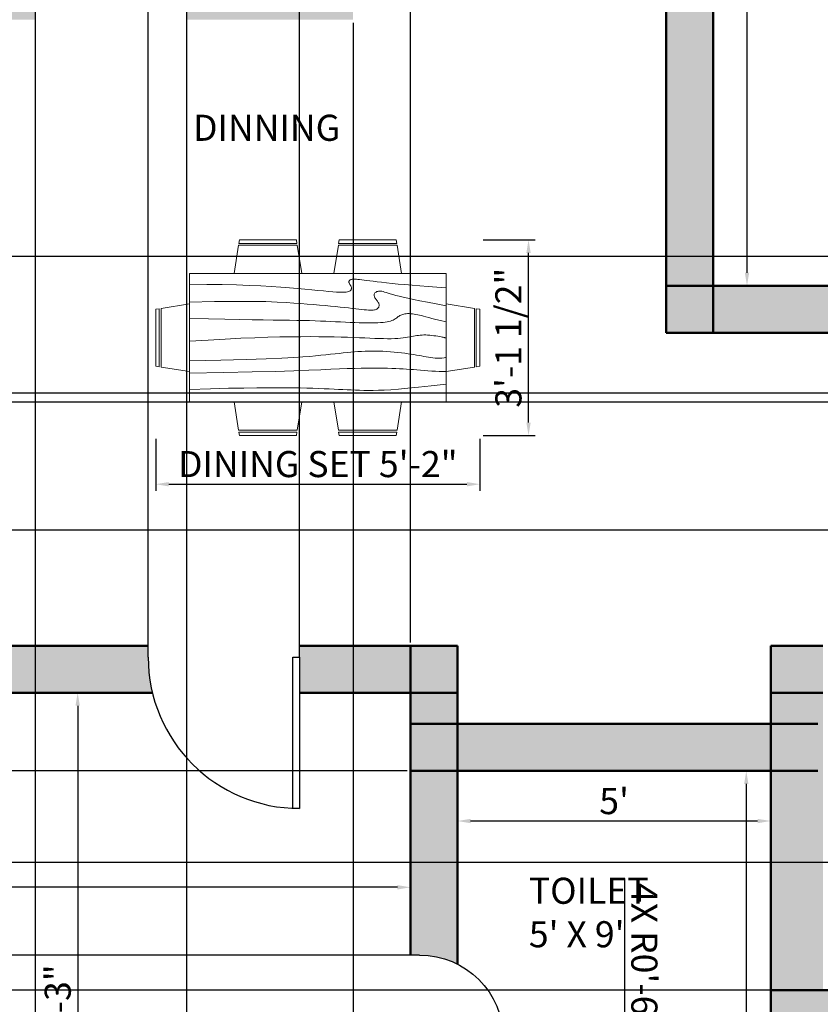
# Model space of a CAD drawing. Units: millimetres. Extents: x 2976 to 3516, y 849 to 1445.
# Tile 4 of 7: x 3119 to 3272, y 1081 to 1270. Entities that reach past the tile are written whole.
import ezdxf

# ---------------------------------------------------------------- set-up
doc = ezdxf.new("R2010")
doc.units = ezdxf.units.MM
for name, color, linetype, lineweight in [('A-AREA-IDEN', 150, 'Continuous', 25), ('A-WALL-PATT', 3, 'Continuous', 13), ('dimensions', 50, 'Continuous', 18), ('doors', 190, 'Continuous', 25), ('furniture', 130, 'Continuous', 18), ('walls', 80, 'Continuous', 50)]:
    doc.layers.add(name, color=color, linetype=linetype, lineweight=lineweight)
doc.styles.get("Standard").update_dxf_attribs({"font": 'arial.ttf'})
doc.dimstyles.new('ISO-25', dxfattribs={"dimtxt": 5, "dimasz": 2.5, "dimexe": 1.25, "dimexo": 0.625, "dimtad": 1, "dimdec": 0, "dimlunit": 3, "dimtxsty": 'Standard', "dimcen": 2.5, "dimadec": 0, "dimazin": 0, "dimtfac": 1, "dimtdec": 0, "dimtmove": 0, "dimatfit": 3, "dimfxl": 1, "dimarcsym": 0})

# ---------------------------------------------------------------- blocks, each defined once
blk = doc.blocks.new('*U2')
for p, q in [((0, 0), (0, -6)), ((40, 0), (40, -6))]:
    blk.add_line(p, q)
blk.add_lwpolyline([(0, 0), (0, 40), (1.75, 40), (1.75, 0)], close=True)
blk.add_arc((0, 0), 40, 0, 90)
blk = doc.blocks.new('Dining Set - 36 x 72 in.')
for p, q in [((-22.2343, 26.00059), (-23.4847, 17.99762)), ((-22.2304, 26), (-5.7608, 26)), ((-22, 27.5), (-22.1562, 26.50042)), ((-5.8416, 26.5), (-22.1534, 26.5)), ((-22, 27.5), (-6, 27.5)), ((-5.8437, 26.49966), (-6, 27.5)), ((-4.5152, 17.99762), (-5.7655, 25.99926)), ((5.7657, 26.00059), (4.5153, 17.99762)), ((5.7696, 26), (22.2392, 26)), ((6, 27.5), (5.8438, 26.50042)), ((22.1584, 26.5), (5.8466, 26.5)), ((6, 27.5), (22, 27.5)), ((22.1563, 26.49966), (22, 27.5)), ((23.4848, 17.99762), (22.2345, 25.99926)), ((36, 18), (-36, 18)), ((-36, 18), (-36, -18)), ((36, -18), (36, 18)), ((-44.0006, 8.23428), (-35.9976, 9.48474)), ((44.0006, 8.23428), (35.9976, 9.48474)), ((-45.5, 8), (-44.5004, 8.15617)), ((-45.5, 8), (-45.5, -8)), ((-44.5, -8.15843), (-44.5, 8.15338)), ((-44, 8.23041), (-44, -8.23915)), ((44, 8.23041), (44, -8.23915)), ((44.5, -8.15843), (44.5, 8.15338)), ((45.5, 8), (44.5005, 8.15617)), ((45.5, 8), (45.5, -8)), ((-44.4997, -8.15631), (-45.5, -8)), ((-35.9976, -9.48476), (-43.9993, -8.2345)), ((35.9976, -9.48476), (43.9993, -8.2345)), ((44.4997, -8.15631), (45.5, -8)), ((-36, -18), (36, -18)), ((-22.2343, -26.0006), (-23.4847, -17.99762)), ((-4.5152, -17.99762), (-5.7655, -25.99928)), ((5.7657, -26.0006), (4.5153, -17.99762)), ((23.4848, -17.99762), (22.2345, -25.99928)), ((-22.2304, -26), (-5.7608, -26)), ((-22, -27.5), (-22.1562, -26.50044)), ((-5.8416, -26.5), (-22.1534, -26.5)), ((-22, -27.5), (-6, -27.5)), ((-5.8437, -26.49967), (-6, -27.5)), ((5.7696, -26), (22.2392, -26)), ((6, -27.5), (5.8438, -26.50044)), ((22.1584, -26.5), (5.8466, -26.5)), ((6, -27.5), (22, -27.5)), ((22.1563, -26.49967), (22, -27.5))]:
    blk.add_line(p, q)
for points in [[(-36, 15), (-31.1772, 14.97754), (-26.8079, 14.91406), (-22.8538, 14.81543), (-19.276, 14.6875), (-16.0362, 14.53613), (-13.0957, 14.36718), (-10.4159, 14.18652), (-7.9583, 14), (-5.6904, 13.81315), (-3.6035, 13.63021), (-1.6954, 13.45508), (0.0365, 13.29166), (1.5945, 13.14388), (2.9811, 13.01562), (4.1988, 12.9108), (5.25, 12.83333), (6.1393, 12.78613), (6.8802, 12.76823), (7.4883, 12.77767), (7.9792, 12.8125), (8.3685, 12.87077), (8.6719, 12.95052), (8.9049, 13.0498), (9.0833, 13.16666), (9.2205, 13.29899), (9.3216, 13.44401), (9.3895, 13.59879), (9.4271, 13.76041), (9.4373, 13.92594), (9.4232, 14.09245), (9.3875, 14.257), (9.3333, 14.41666), (9.2638, 14.56917), (9.1836, 14.71484), (9.0975, 14.85465), (9.0104, 14.98958), (8.9272, 15.1206), (8.8529, 15.2487), (8.7922, 15.37483), (8.75, 15.5), (8.7305, 15.62467), (8.7344, 15.74739), (8.7617, 15.86621), (8.8125, 15.97916), (8.8867, 16.08431), (8.9844, 16.17968), (9.1055, 16.26334), (9.25, 16.33333), (9.4189, 16.38802), (9.6172, 16.42708), (9.8506, 16.45052), (10.125, 16.45833), (10.4463, 16.45052), (10.8203, 16.42708), (11.2529, 16.38802), (11.75, 16.33333), (12.3184, 16.26318), (12.9694, 16.17838), (13.7151, 16.07991), (14.5677, 15.96875), (15.5395, 15.84586), (16.6426, 15.71224), (17.8893, 15.56884), (19.2917, 15.41666), (20.859, 15.25667), (22.5879, 15.08984), (24.4721, 14.91715), (26.5052, 14.73958), (28.6809, 14.5581), (30.9929, 14.3737), (33.4347, 14.18733), (36, 14)], [(-36, 10), (-28.9766, 10.14274), (-23.1725, 10.20442), (-18.4241, 10.19775), (-14.5677, 10.13541), (-11.4399, 10.03011), (-8.877, 9.89453), (-6.7154, 9.74137), (-4.7917, 9.58333), (-2.9698, 9.43082), (-1.2246, 9.28515), (0.4415, 9.14534), (2.026, 9.01041), (3.5266, 8.87939), (4.9408, 8.7513), (6.266, 8.62516), (7.5, 8.5), (8.6411, 8.37549), (9.6914, 8.2539), (10.6538, 8.13818), (11.5312, 8.03125), (12.3267, 7.93603), (13.043, 7.85547), (13.6831, 7.79248), (14.25, 7.75), (14.7471, 7.7303), (15.1797, 7.73307), (15.5537, 7.75732), (15.875, 7.80208), (16.1494, 7.86637), (16.3828, 7.94922), (16.5811, 8.04964), (16.75, 8.16666), (16.8944, 8.29915), (17.0143, 8.44531), (17.1089, 8.60319), (17.1771, 8.77083), (17.218, 8.94629), (17.2305, 9.1276), (17.2137, 9.31282), (17.1667, 9.5), (17.0895, 9.6875), (16.987, 9.875), (16.8649, 10.0625), (16.7292, 10.25), (16.5856, 10.4375), (16.4401, 10.625), (16.2985, 10.8125), (16.1667, 11), (16.05, 11.18733), (15.9518, 11.3737), (15.8752, 11.5581), (15.8229, 11.73958), (15.798, 11.91715), (15.8034, 12.08984), (15.842, 12.25667), (15.9167, 12.41666), (16.0295, 12.56836), (16.1784, 12.70833), (16.3605, 12.83268), (16.5729, 12.9375), (16.8127, 13.01888), (17.0768, 13.07291), (17.3625, 13.0957), (17.6667, 13.08333), (17.9894, 13.03312), (18.3418, 12.94726), (18.7382, 12.82918), (19.1927, 12.68229), (19.7195, 12.51001), (20.3327, 12.31575), (21.0465, 12.10294), (21.875, 11.875), (22.8357, 11.63354), (23.959, 11.37304), (25.2786, 11.08618), (26.8282, 10.76562), (28.6414, 10.40405), (30.752, 9.99414), (33.1936, 9.52856), (36, 9)], [(-36, 5.5), (-30.7157, 5.3348), (-26.069, 5.20963), (-21.9946, 5.11767), (-18.4271, 5.05208), (-15.3009, 5.00602), (-12.5508, 4.97265), (-10.1112, 4.94515), (-7.9167, 4.91666), (-5.909, 4.88167), (-4.0586, 4.83984), (-2.3429, 4.79215), (-0.7396, 4.73958), (0.7739, 4.6831), (2.22, 4.6237), (3.6213, 4.56233), (5, 4.5), (6.373, 4.43782), (7.7344, 4.3776), (9.0723, 4.32129), (10.375, 4.27083), (11.6309, 4.22819), (12.8281, 4.19531), (13.9551, 4.17415), (15, 4.16666), (15.954, 4.17448), (16.819, 4.19791), (17.6001, 4.23698), (18.3021, 4.29166), (18.9299, 4.36198), (19.4883, 4.44791), (19.9823, 4.54948), (20.4167, 4.66666), (20.7969, 4.79899), (21.1302, 4.94401), (21.4245, 5.09879), (21.6875, 5.26041), (21.9271, 5.42594), (22.1511, 5.59245), (22.3672, 5.757), (22.5834, 5.91666), (22.8065, 6.06868), (23.0404, 6.21093), (23.2879, 6.34147), (23.5521, 6.45833), (23.8358, 6.55957), (24.142, 6.64323), (24.4735, 6.70735), (24.8334, 6.75), (25.2235, 6.76969), (25.642, 6.76692), (26.0858, 6.74267), (26.5521, 6.69791), (27.0379, 6.63362), (27.5404, 6.55078), (28.0565, 6.45036), (28.5834, 6.33333), (29.1242, 6.19987), (29.7071, 6.04687), (30.3661, 5.87044), (31.1354, 5.66666), (32.0493, 5.43164), (33.142, 5.16146), (34.4475, 4.85221), (36, 4.5)], [(-36, -1), (-30.7915, -0.6591), (-26.0195, -0.38216), (-21.6519, -0.16284), (-17.6563, 0.00521), (-14.0005, 0.12833), (-10.6523, 0.21289), (-7.5796, 0.26522), (-4.75, 0.29166), (-2.134, 0.29793), (0.2878, 0.28711), (2.5317, 0.26163), (4.6146, 0.22396), (6.5529, 0.17651), (8.3633, 0.12174), (10.0623, 0.06209), (11.6667, 0), (13.1899, -0.06201), (14.6341, -0.1211), (15.9982, -0.17432), (17.2813, -0.21875), (18.4823, -0.25147), (19.6003, -0.26953), (20.6343, -0.27002), (21.5834, -0.25), (22.4481, -0.20768), (23.2357, -0.14584), (23.9549, -0.06836), (24.6146, 0.02083), (25.2235, 0.11784), (25.7904, 0.21875), (26.3241, 0.31966), (26.8334, 0.41666), (27.3265, 0.50618), (27.8099, 0.58593), (28.2894, 0.65397), (28.7709, 0.70833), (29.2601, 0.74707), (29.763, 0.76823), (30.2855, 0.76985), (30.8334, 0.75), (31.4088, 0.70784), (31.9994, 0.64713), (32.589, 0.57275), (33.1615, 0.48958), (33.7008, 0.4025), (34.1908, 0.3164), (34.6153, 0.23616), (34.9584, 0.16666), (35.2099, 0.11165), (35.3848, 0.07031), (35.504, 0.04069), (35.5886, 0.02083), (35.6594, 0.00879), (35.7377, 0.0026), (35.8442, 0.00032), (36, 0)], [(-36, -6.5), (-27.1843, -6.31267), (-20.084, -6.1263), (-14.469, -5.9419), (-10.1094, -5.76042), (-6.7752, -5.58285), (-4.2363, -5.41016), (-2.2629, -5.24333), (-0.625, -5.08334), (0.8708, -4.93099), (2.2715, -4.78646), (3.5872, -4.64974), (4.8281, -4.52084), (6.0046, -4.39974), (7.127, -4.28646), (8.2053, -4.18099), (9.25, -4.08334), (10.2705, -3.99382), (11.2734, -3.91407), (12.2647, -3.84603), (13.25, -3.79167), (14.2354, -3.75293), (15.2266, -3.73177), (16.2295, -3.73015), (17.25, -3.75), (18.2912, -3.79248), (19.3451, -3.85547), (20.4009, -3.93604), (21.4479, -4.03125), (22.4754, -4.13819), (23.4727, -4.25391), (24.4289, -4.37549), (25.3334, -4.5), (26.1785, -4.62492), (26.9694, -4.74935), (27.7145, -4.87281), (28.4219, -4.99479), (29.1, -5.11483), (29.7572, -5.23242), (30.4016, -5.34709), (31.0417, -5.45834), (31.6837, -5.56437), (32.3262, -5.65821), (32.9658, -5.73153), (33.599, -5.77604), (34.2224, -5.78345), (34.8327, -5.74545), (35.4264, -5.65373), (36, -5.5)], [(-36, -10), (-26.4022, -9.81299), (-18.4675, -9.62891), (-11.9839, -9.45069), (-6.7396, -9.28125), (-2.5226, -9.12354), (0.8789, -8.98047), (3.6769, -8.85498), (6.0833, -8.75), (8.2767, -8.66765), (10.3021, -8.60677), (12.1712, -8.56543), (13.8958, -8.54167), (15.4876, -8.53353), (16.9583, -8.53907), (18.3197, -8.55632), (19.5834, -8.58334), (20.7616, -8.61841), (21.8685, -8.66081), (22.9188, -8.71004), (23.9271, -8.76563), (24.9081, -8.82707), (25.8763, -8.89388), (26.8465, -8.96558), (27.8334, -9.04167), (28.8474, -9.12118), (29.8828, -9.20117), (30.93, -9.27824), (31.9792, -9.34896), (33.0205, -9.40991), (34.0443, -9.45768), (35.0407, -9.48885), (36, -9.5)], [(-36, -14.5), (-30.0881, -14.33513), (-25.0332, -14.21224), (-20.7312, -14.12647), (-17.0781, -14.07292), (-13.97, -14.04671), (-11.3027, -14.04297), (-8.9724, -14.05681), (-6.875, -14.08334), (-4.9224, -14.11833), (-3.0905, -14.16016), (-1.3709, -14.20785), (0.2448, -14.26042), (1.7647, -14.3169), (3.1973, -14.3763), (4.5507, -14.43767), (5.8333, -14.5), (7.0554, -14.5621), (8.235, -14.62175), (9.3922, -14.67652), (10.5469, -14.72396), (11.7192, -14.76164), (12.929, -14.78711), (14.1965, -14.79794), (15.5417, -14.79167), (16.9933, -14.76424), (18.6152, -14.70508), (20.4804, -14.60197), (22.6615, -14.44271), (25.2312, -14.21509), (28.2624, -13.9069), (31.8277, -13.50594), (36, -13)]]:
    blk.add_lwpolyline(points)
blk = doc.blocks.new('*D14')
at = {"layer": 'Defpoints', "color": 0, "transparency": 16777216}
for p in [(3258.13, 1398.88), (3258.13, 1218.88), (3258.13, 1218.88)]:
    blk.add_point(p, dxfattribs=at)
at = {"layer": 'dimensions', "color": 0, "lineweight": -2, "transparency": 16777216}
for p, q in [((3258.76, 1398.88), (3259.38, 1398.88)), ((3258.13, 1396.38), (3258.13, 1221.38)), ((3258.76, 1218.88), (3259.38, 1218.88))]:
    blk.add_line(p, q, dxfattribs=at)
at = {"layer": 'dimensions', "color": 0, "transparency": 16777216}
for points in [[(3257.72, 1396.38), (3258.55, 1396.38), (3258.13, 1398.88)], [(3257.72, 1221.38), (3258.55, 1221.38), (3258.13, 1218.88)]]:
    blk.add_solid(points, dxfattribs=at)
at = {"layer": 'dimensions', "color": 0, "transparency": 16777216, "insert": (3254.96, 1308.88), "char_height": 5, "attachment_point": 5, "rotation": 90}
blk.add_mtext("15'", dxfattribs=at)
blk = doc.blocks.new('*D15')
at = {"layer": 'Defpoints', "color": 0, "transparency": 16777216}
for p in [(3022.67, 1108.78), (3193.67, 1108.78), (3022.67, 1103.57)]:
    blk.add_point(p, dxfattribs=at)
at = {"layer": 'dimensions', "color": 0, "lineweight": -2, "transparency": 16777216}
for p, q in [((3022.67, 1108.16), (3022.67, 1102.32)), ((3193.67, 1108.16), (3193.67, 1102.32)), ((3191.17, 1103.57), (3025.17, 1103.57))]:
    blk.add_line(p, q, dxfattribs=at)
at = {"layer": 'dimensions', "color": 0, "transparency": 16777216}
for points in [[(3025.17, 1103.99), (3025.17, 1103.16), (3022.67, 1103.57)], [(3191.17, 1103.99), (3191.17, 1103.16), (3193.67, 1103.57)]]:
    blk.add_solid(points, dxfattribs=at)
at = {"layer": 'dimensions', "color": 0, "transparency": 16777216, "insert": (3108.17, 1106.75), "char_height": 5, "attachment_point": 5}
blk.add_mtext('14\'-3"', dxfattribs=at)
blk = doc.blocks.new('*D16')
at = {"layer": 'Defpoints', "color": 0, "transparency": 16777216}
for p in [(3129.91, 1140.88), (3129.91, 1017.88), (3129.91, 1017.88)]:
    blk.add_point(p, dxfattribs=at)
at = {"layer": 'dimensions', "color": 0, "lineweight": -2, "transparency": 16777216}
for p, q in [((3130.53, 1140.88), (3131.16, 1140.88)), ((3129.91, 1138.38), (3129.91, 1020.38)), ((3130.53, 1017.88), (3131.16, 1017.88))]:
    blk.add_line(p, q, dxfattribs=at)
at = {"layer": 'dimensions', "color": 0, "transparency": 16777216}
for points in [[(3129.49, 1138.38), (3130.32, 1138.38), (3129.91, 1140.88)], [(3129.49, 1020.38), (3130.32, 1020.38), (3129.91, 1017.88)]]:
    blk.add_solid(points, dxfattribs=at)
at = {"layer": 'dimensions', "color": 0, "transparency": 16777216, "insert": (3126.73, 1079.38), "char_height": 5, "attachment_point": 5, "rotation": 90}
blk.add_mtext('10\'-3"', dxfattribs=at)
blk = doc.blocks.new('*D19')
at = {"layer": 'Defpoints', "color": 0, "transparency": 16777216}
for p in [(3257.99, 1125.88), (3257.99, 1017.88), (3257.99, 1017.88)]:
    blk.add_point(p, dxfattribs=at)
at = {"layer": 'dimensions', "color": 0, "lineweight": -2, "transparency": 16777216}
for p, q in [((3258.62, 1125.88), (3259.24, 1125.88)), ((3257.99, 1123.38), (3257.99, 1020.38)), ((3258.62, 1017.88), (3259.24, 1017.88))]:
    blk.add_line(p, q, dxfattribs=at)
at = {"layer": 'dimensions', "color": 0, "transparency": 16777216}
for points in [[(3257.58, 1123.38), (3258.41, 1123.38), (3257.99, 1125.88)], [(3257.58, 1020.38), (3258.41, 1020.38), (3257.99, 1017.88)]]:
    blk.add_solid(points, dxfattribs=at)
at = {"layer": 'dimensions', "color": 0, "transparency": 16777216, "insert": (3254.82, 1071.88), "char_height": 5, "attachment_point": 5, "rotation": 90}
blk.add_mtext("9'", dxfattribs=at)
blk = doc.blocks.new('*D20')
at = {"layer": 'Defpoints', "color": 0, "transparency": 16777216}
for p in [(3202.67, 1119.36), (3262.67, 1119.68), (3202.67, 1116.28)]:
    blk.add_point(p, dxfattribs=at)
at = {"layer": 'dimensions', "color": 0, "lineweight": -2, "transparency": 16777216}
for p, q in [((3202.67, 1118.74), (3202.67, 1115.03)), ((3262.67, 1119.06), (3262.67, 1115.03)), ((3260.17, 1116.28), (3205.17, 1116.28))]:
    blk.add_line(p, q, dxfattribs=at)
at = {"layer": 'dimensions', "color": 0, "transparency": 16777216}
for points in [[(3205.17, 1116.69), (3205.17, 1115.86), (3202.67, 1116.28)], [(3260.17, 1116.69), (3260.17, 1115.86), (3262.67, 1116.28)]]:
    blk.add_solid(points, dxfattribs=at)
at = {"layer": 'dimensions', "color": 0, "transparency": 16777216, "insert": (3232.67, 1119.45), "char_height": 5, "attachment_point": 5}
blk.add_mtext("5'", dxfattribs=at)
blk = doc.blocks.new('*D36')
at = {"layer": 'Defpoints', "color": 0, "transparency": 16777216}
for p in [(3144.86, 1190.16), (3206.96, 1190.16), (3206.96, 1180.84)]:
    blk.add_point(p, dxfattribs=at)
at = {"layer": 'dimensions', "color": 0, "lineweight": -2, "transparency": 16777216}
for p, q in [((3144.86, 1189.53), (3144.86, 1179.59)), ((3206.96, 1189.53), (3206.96, 1179.59)), ((3147.36, 1180.84), (3204.46, 1180.84))]:
    blk.add_line(p, q, dxfattribs=at)
at = {"layer": 'dimensions', "color": 0, "transparency": 16777216}
for points in [[(3147.36, 1181.26), (3147.36, 1180.42), (3144.86, 1180.84)], [(3204.46, 1181.26), (3204.46, 1180.42), (3206.96, 1180.84)]]:
    blk.add_solid(points, dxfattribs=at)
at = {"layer": 'dimensions', "color": 0, "transparency": 16777216, "insert": (3175.91, 1184.05), "char_height": 5, "attachment_point": 5}
blk.add_mtext('DINING SET 5\'-2"', dxfattribs=at)
blk = doc.blocks.new('*D37')
at = {"layer": 'Defpoints', "color": 0, "transparency": 16777216}
for p in [(3206.96, 1227.69), (3216.28, 1227.69), (3206.96, 1190.16)]:
    blk.add_point(p, dxfattribs=at)
at = {"layer": 'dimensions', "color": 0, "lineweight": -2, "transparency": 16777216}
for p, q in [((3207.59, 1227.69), (3217.53, 1227.69)), ((3216.28, 1192.66), (3216.28, 1225.19)), ((3207.59, 1190.16), (3217.53, 1190.16))]:
    blk.add_line(p, q, dxfattribs=at)
at = {"layer": 'dimensions', "color": 0, "transparency": 16777216}
for points in [[(3215.86, 1225.19), (3216.69, 1225.19), (3216.28, 1227.69)], [(3215.86, 1192.66), (3216.69, 1192.66), (3216.28, 1190.16)]]:
    blk.add_solid(points, dxfattribs=at)
at = {"layer": 'dimensions', "color": 0, "transparency": 16777216, "insert": (3213.07, 1208.92), "char_height": 5, "attachment_point": 5, "rotation": 90}
blk.add_mtext('3\'-1 1/2"', dxfattribs=at)
blk = doc.blocks.new('*D44')
at = {"layer": 'Defpoints', "color": 0, "transparency": 16777216}
for p in [(3242.67, 1434.42), (3091.67, 1224.53), (3242.67, 1209.88)]:
    blk.add_point(p, dxfattribs=at)
at = {"layer": 'dimensions', "color": 0, "lineweight": -2, "transparency": 16777216}
for p, q in [((3091.67, 1225.16), (3091.67, 1435.67)), ((3094.17, 1434.42), (3240.17, 1434.42)), ((3242.67, 1210.51), (3242.67, 1435.67))]:
    blk.add_line(p, q, dxfattribs=at)
at = {"layer": 'dimensions', "color": 0, "transparency": 16777216}
for points in [[(3094.17, 1434.84), (3094.17, 1434), (3091.67, 1434.42)], [(3240.17, 1434.84), (3240.17, 1434), (3242.67, 1434.42)]]:
    blk.add_solid(points, dxfattribs=at)
at = {"layer": 'dimensions', "color": 0, "transparency": 16777216, "insert": (3167.17, 1437.56), "char_height": 5, "attachment_point": 5}
blk.add_mtext('12\'-7"', dxfattribs=at)
blk = doc.blocks.new('*D52')
at = {"layer": 'Defpoints', "color": 0, "transparency": 16777216}
for p in [(3121.76, 1269.88), (3150.74, 1269.88), (3150.74, 853.34)]:
    blk.add_point(p, dxfattribs=at)
at = {"layer": 'dimensions', "color": 0, "lineweight": -2, "transparency": 16777216}
for p, q in [((3121.76, 1269.26), (3121.76, 852.09)), ((3150.74, 1269.26), (3150.74, 852.09)), ((3124.26, 853.34), (3148.24, 853.34))]:
    blk.add_line(p, q, dxfattribs=at)
at = {"layer": 'dimensions', "color": 0, "transparency": 16777216}
for points in [[(3124.26, 853.76), (3124.26, 852.92), (3121.76, 853.34)], [(3148.24, 853.76), (3148.24, 852.92), (3150.74, 853.34)]]:
    blk.add_solid(points, dxfattribs=at)
at = {"layer": 'dimensions', "color": 0, "transparency": 16777216, "insert": (3136.25, 856.52), "char_height": 5, "attachment_point": 5}
blk.add_mtext('2\'-5"', dxfattribs=at)
blk = doc.blocks.new('*D53')
at = {"layer": 'Defpoints', "color": 0, "transparency": 16777216}
for p in [(2987.13, 1090.58), (3193.67, 1090.58), (3193.67, 1074.53)]:
    blk.add_point(p, dxfattribs=at)
at = {"layer": 'dimensions', "color": 0, "lineweight": -2, "transparency": 16777216}
for p, q in [((3193.05, 1090.58), (2985.88, 1090.58)), ((2987.13, 1077.03), (2987.13, 1088.08)), ((3193.05, 1074.53), (2985.88, 1074.53))]:
    blk.add_line(p, q, dxfattribs=at)
at = {"layer": 'dimensions', "color": 0, "transparency": 16777216}
for points in [[(2986.71, 1088.08), (2987.55, 1088.08), (2987.13, 1090.58)], [(2986.71, 1077.03), (2987.55, 1077.03), (2987.13, 1074.53)]]:
    blk.add_solid(points, dxfattribs=at)
at = {"layer": 'dimensions', "color": 0, "transparency": 16777216, "insert": (2984, 1082.56), "char_height": 5, "attachment_point": 5, "rotation": 90}
blk.add_mtext('1\'-4"', dxfattribs=at)
blk = doc.blocks.new('*D54')
at = {"layer": 'Defpoints', "color": 0, "transparency": 16777216}
for p in [(3172.4, 1434.42), (3143.42, 1149.88), (3172.4, 1149.88)]:
    blk.add_point(p, dxfattribs=at)
at = {"layer": 'dimensions', "color": 0, "lineweight": -2, "transparency": 16777216}
for p, q in [((3143.42, 1150.51), (3143.42, 1435.67)), ((3145.92, 1434.42), (3169.9, 1434.42)), ((3172.4, 1150.51), (3172.4, 1435.67))]:
    blk.add_line(p, q, dxfattribs=at)
at = {"layer": 'dimensions', "color": 0, "transparency": 16777216}
for points in [[(3145.92, 1434.84), (3145.92, 1434), (3143.42, 1434.42)], [(3169.9, 1434.84), (3169.9, 1434), (3172.4, 1434.42)]]:
    blk.add_solid(points, dxfattribs=at)
at = {"layer": 'dimensions', "color": 0, "transparency": 16777216, "insert": (3157.91, 1437.6), "char_height": 5, "attachment_point": 5}
blk.add_mtext('2\'-5"', dxfattribs=at)
blk = doc.blocks.new('*D63')
at = {"layer": 'Defpoints', "color": 0, "transparency": 16777216}
for p in [(2987.13, 1196.55), (3364.14, 1196.55), (3364.14, 1172.02)]:
    blk.add_point(p, dxfattribs=at)
at = {"layer": 'dimensions', "color": 0, "lineweight": -2, "transparency": 16777216}
for p, q in [((2987.13, 1196.55), (2987.13, 1225.33)), ((3363.51, 1196.55), (2985.88, 1196.55)), ((2987.13, 1174.52), (2987.13, 1194.05)), ((3363.51, 1172.02), (2985.88, 1172.02))]:
    blk.add_line(p, q, dxfattribs=at)
at = {"layer": 'dimensions', "color": 0, "transparency": 16777216}
for points in [[(2986.71, 1194.05), (2987.55, 1194.05), (2987.13, 1196.55)], [(2986.71, 1174.52), (2987.55, 1174.52), (2987.13, 1172.02)]]:
    blk.add_solid(points, dxfattribs=at)
at = {"layer": 'dimensions', "color": 0, "transparency": 16777216, "insert": (2983.92, 1212.19), "char_height": 5, "attachment_point": 5, "rotation": 90}
blk.add_mtext('2\'-0 1/2"', dxfattribs=at)
blk = doc.blocks.new('*D67')
at = {"layer": 'Defpoints', "color": 0, "transparency": 16777216}
for p in [(2987.13, 1108.35), (3300.46, 1108.35), (3300.46, 1083.88)]:
    blk.add_point(p, dxfattribs=at)
at = {"layer": 'dimensions', "color": 0, "lineweight": -2, "transparency": 16777216}
for p, q in [((2987.13, 1108.35), (2987.13, 1137.13)), ((3299.83, 1108.35), (2985.88, 1108.35)), ((2987.13, 1086.38), (2987.13, 1105.85)), ((3299.83, 1083.88), (2985.88, 1083.88))]:
    blk.add_line(p, q, dxfattribs=at)
at = {"layer": 'dimensions', "color": 0, "transparency": 16777216}
for points in [[(2986.71, 1105.85), (2987.55, 1105.85), (2987.13, 1108.35)], [(2986.71, 1086.38), (2987.55, 1086.38), (2987.13, 1083.88)]]:
    blk.add_solid(points, dxfattribs=at)
at = {"layer": 'dimensions', "color": 0, "transparency": 16777216, "insert": (2983.92, 1123.99), "char_height": 5, "attachment_point": 5, "rotation": 90}
blk.add_mtext('2\'-0 1/2"', dxfattribs=at)
blk = doc.blocks.new('*D71')
at = {"layer": 'Defpoints', "color": 0, "transparency": 16777216}
for p in [(2987.13, 1125.88), (3193.67, 1125.88), (3193.67, 1090.58)]:
    blk.add_point(p, dxfattribs=at)
at = {"layer": 'dimensions', "color": 0, "lineweight": -2, "transparency": 16777216}
for p, q in [((3193.05, 1125.88), (2985.88, 1125.88)), ((2987.13, 1093.08), (2987.13, 1123.38)), ((3193.05, 1090.58), (2985.88, 1090.58))]:
    blk.add_line(p, q, dxfattribs=at)
at = {"layer": 'dimensions', "color": 0, "transparency": 16777216}
for points in [[(2986.71, 1123.38), (2987.55, 1123.38), (2987.13, 1125.88)], [(2986.71, 1093.08), (2987.55, 1093.08), (2987.13, 1090.58)]]:
    blk.add_solid(points, dxfattribs=at)
at = {"layer": 'dimensions', "color": 0, "transparency": 16777216, "insert": (2983.92, 1108.23), "char_height": 5, "attachment_point": 5, "rotation": 90}
blk.add_mtext('2\'-11 1/2"', dxfattribs=at)
blk = doc.blocks.new('*D72')
at = {"layer": 'Defpoints', "color": 0, "transparency": 16777216}
for p in [(3150.74, 1269.88), (3182.67, 1269.88), (3182.67, 853.34)]:
    blk.add_point(p, dxfattribs=at)
at = {"layer": 'dimensions', "color": 0, "lineweight": -2, "transparency": 16777216}
for p, q in [((3150.74, 1269.26), (3150.74, 852.09)), ((3182.67, 1269.26), (3182.67, 852.09)), ((3153.24, 853.34), (3180.17, 853.34))]:
    blk.add_line(p, q, dxfattribs=at)
at = {"layer": 'dimensions', "color": 0, "transparency": 16777216}
for points in [[(3153.24, 853.76), (3153.24, 852.92), (3150.74, 853.34)], [(3180.17, 853.76), (3180.17, 852.92), (3182.67, 853.34)]]:
    blk.add_solid(points, dxfattribs=at)
at = {"layer": 'dimensions', "color": 0, "transparency": 16777216, "insert": (3166.71, 856.52), "char_height": 5, "attachment_point": 5}
blk.add_mtext('2\'-8"', dxfattribs=at)
blk = doc.blocks.new('*D73')
at = {"layer": 'Defpoints', "color": 0, "transparency": 16777216}
for p in [(3193.67, 1434.42), (3172.4, 1149.88), (3193.67, 1149.88)]:
    blk.add_point(p, dxfattribs=at)
at = {"layer": 'dimensions', "color": 0, "lineweight": -2, "transparency": 16777216}
for p, q in [((3172.4, 1150.51), (3172.4, 1435.67)), ((3174.9, 1434.42), (3191.17, 1434.42)), ((3193.67, 1150.51), (3193.67, 1435.67)), ((3193.67, 1434.42), (3221.89, 1434.42))]:
    blk.add_line(p, q, dxfattribs=at)
at = {"layer": 'dimensions', "color": 0, "transparency": 16777216}
for points in [[(3174.9, 1434.84), (3174.9, 1434), (3172.4, 1434.42)], [(3191.17, 1434.84), (3191.17, 1434), (3193.67, 1434.42)]]:
    blk.add_solid(points, dxfattribs=at)
at = {"layer": 'dimensions', "color": 0, "transparency": 16777216, "insert": (3209.03, 1437.63), "char_height": 5, "attachment_point": 5}
blk.add_mtext('1\'-9 1/2"', dxfattribs=at)
blk = doc.blocks.new('*D83')
at = {"layer": 'Defpoints', "color": 0, "transparency": 16777216}
for p in [(3091.67, 1224.53), (3512.21, 1224.53), (3091.67, 1198.35)]:
    blk.add_point(p, dxfattribs=at)
at = {"layer": 'dimensions', "color": 0, "lineweight": -2, "transparency": 16777216}
for p, q in [((3092.3, 1224.53), (3513.46, 1224.53)), ((3512.21, 1200.85), (3512.21, 1222.03)), ((3092.3, 1198.35), (3513.46, 1198.35))]:
    blk.add_line(p, q, dxfattribs=at)
at = {"layer": 'dimensions', "color": 0, "transparency": 16777216}
for points in [[(3511.79, 1222.03), (3512.63, 1222.03), (3512.21, 1224.53)], [(3511.79, 1200.85), (3512.63, 1200.85), (3512.21, 1198.35)]]:
    blk.add_solid(points, dxfattribs=at)
at = {"layer": 'dimensions', "color": 0, "transparency": 16777216, "insert": (3509.08, 1211.44), "char_height": 5, "attachment_point": 5, "rotation": 90}
blk.add_mtext('2\'-2"', dxfattribs=at)
blk = doc.blocks.new('*D88')
at = {"layer": 'Defpoints', "color": 0, "transparency": 16777216}
for p in [(3234.64, 1069.96), (3234.64, 1063.98)]:
    blk.add_point(p, dxfattribs=at)
at = {"layer": 'dimensions', "color": 0, "lineweight": -2, "transparency": 16777216}
for p, q in [((3234.64, 1105.24), (3234.64, 1072.46)), ((3234.64, 1063.98), (3234.64, 1069.96))]:
    blk.add_line(p, q, dxfattribs=at)
at = {"layer": 'dimensions', "color": 0, "transparency": 16777216}
blk.add_solid([(3235.06, 1072.46), (3234.22, 1072.46), (3234.64, 1069.96)], dxfattribs=at)
at = {"layer": 'dimensions', "color": 0, "transparency": 16777216, "insert": (3237.82, 1090.1), "char_height": 5, "attachment_point": 5, "rotation": 270.0033}
blk.add_mtext('4X R0\'-6"', dxfattribs=at)

msp = doc.modelspace()

# ---------------------------------------------------------------- hatches: boundary and pattern name
at = {"layer": 'A-WALL-PATT'}
h = msp.add_hatch(color=256, dxfattribs=at)
h.dxf.hatch_style = 1
h.paths.add_polyline_path([(3022.67, 1398.88), (3013.67, 1398.88), (3013.67, 1278.88), (3022.67, 1278.88)])
h.paths.add_polyline_path([(3082.67, 1278.88), (3022.67, 1278.88), (3022.67, 1269.88), (3082.67, 1269.88)])
h.paths.add_polyline_path([(3022.67, 1278.88), (3013.67, 1278.88), (3013.67, 1269.88), (3022.67, 1269.88)])
h.paths.add_polyline_path([(3091.67, 1278.88), (3082.67, 1278.88), (3082.67, 1269.88), (3091.67, 1269.88)])
h.paths.add_polyline_path([(3121.76, 1278.88), (3091.67, 1278.88), (3091.67, 1269.88), (3121.76, 1269.88), (3121.76, 1272.56)])
h.paths.add_polyline_path([(3022.67, 1269.88), (3013.67, 1269.88), (3013.67, 1149.88), (3022.67, 1149.88)])
h.paths.add_polyline_path([(3022.67, 1140.88), (3013.67, 1140.88), (3013.67, 1017.88), (3022.67, 1017.88)])
h.paths.add_polyline_path([(3022.67, 1149.88), (3013.67, 1149.88), (3013.67, 1140.88), (3022.67, 1140.88)])
h.paths.add_polyline_path([(3082.67, 1149.88), (3022.67, 1149.88), (3022.67, 1140.88), (3082.67, 1140.88)])
h.paths.add_polyline_path([(3091.67, 1149.88), (3082.67, 1149.88), (3082.67, 1140.88), (3091.67, 1140.88)])
h.paths.add_polyline_path([(3143.42, 1147.68), (3143.42, 1149.88), (3091.67, 1149.88), (3091.67, 1140.88), (3144.23, 1140.88, -0.059251)])
h.paths.add_polyline_path([(3193.67, 1149.88), (3172.4, 1149.88), (3172.4, 1147.68), (3172.4, 1140.88), (3193.67, 1140.88)])
h.paths.add_polyline_path([(3202.67, 1149.88), (3193.67, 1149.88), (3193.67, 1140.88), (3202.67, 1140.88)])
h.paths.add_polyline_path([(3272.67, 1149.88), (3262.67, 1149.88), (3262.67, 1140.88), (3272.67, 1140.88)])
h.paths.add_polyline_path([(3272.67, 1140.88), (3262.67, 1140.88), (3262.67, 1083.88), (3272.67, 1083.88)])
h.paths.add_polyline_path([(3202.67, 1140.88), (3193.67, 1140.88), (3193.67, 1090.58), (3195.4, 1090.58, -0.118064), (3202.67, 1088.84)])
h.paths.add_polyline_path([(3202.67, 1074.53), (3195.4, 1074.53), (3193.67, 1074.53), (3193.67, 1017.88), (3202.67, 1017.88)])
h.paths.add_polyline_path([(3202.67, 1017.88), (3193.67, 1017.88), (3193.67, 1008.88), (3202.67, 1008.88)])
h.paths.add_polyline_path([(3193.67, 1017.88), (3112.23, 1017.88), (3112.23, 1008.88), (3193.67, 1008.88)])
h.paths.add_polyline_path([(3068.25, 1017.88), (3022.67, 1017.88), (3022.67, 1008.88), (3068.25, 1008.88)])
h.paths.add_polyline_path([(3022.67, 1017.88), (3013.67, 1017.88), (3013.67, 1008.88), (3022.67, 1008.88)])
h.paths.add_polyline_path([(3272.67, 1074.88), (3262.67, 1074.88), (3262.67, 1017.88), (3271.67, 1017.88), (3272.67, 1017.88)])
h.paths.add_polyline_path([(3272.67, 1083.88), (3262.67, 1083.88), (3262.67, 1074.88), (3272.67, 1074.88)])
h.paths.add_polyline_path([(3284.41, 1082.91), (3284.41, 1083.88), (3272.67, 1083.88), (3272.67, 1074.88), (3284.41, 1074.88)])
h.paths.add_polyline_path([(3383.67, 1083.88), (3300.46, 1083.88), (3300.46, 1082.91, -0.131652), (3298.31, 1074.88), (3383.67, 1074.88)])
h.paths.add_polyline_path([(3392.67, 1083.88), (3383.67, 1083.88), (3383.67, 1074.88), (3392.67, 1074.88)])
h.paths.add_polyline_path([(3392.67, 1074.88), (3383.67, 1074.88), (3383.67, 1017.88), (3392.67, 1017.88)])
h.paths.add_polyline_path([(3392.67, 1017.88), (3383.67, 1017.88), (3383.67, 1008.88), (3392.67, 1008.88)])
h.paths.add_polyline_path([(3383.67, 1017.88), (3347.17, 1017.88), (3347.17, 1008.88), (3383.67, 1008.88)])
h.paths.add_polyline_path([(3303.78, 1017.88), (3272.67, 1017.88), (3272.67, 1008.88), (3303.78, 1008.88)])
h.paths.add_polyline_path([(3272.67, 1017.88), (3271.67, 1017.88), (3262.67, 1017.88), (3262.67, 1008.88), (3272.67, 1008.88)])
h.paths.add_polyline_path([(3262.67, 1017.88), (3243.44, 1017.88), (3243.44, 1008.88), (3262.67, 1008.88)])
h.paths.add_polyline_path([(3218.58, 1017.88), (3202.67, 1017.88), (3202.67, 1008.88), (3218.58, 1008.88)])
h.paths.add_polyline_path([(3392.67, 1209.88), (3383.67, 1209.88), (3383.67, 1083.88), (3392.67, 1083.88)])
h.paths.add_polyline_path([(3392.67, 1218.88), (3383.67, 1218.88), (3383.67, 1209.88), (3392.67, 1209.88)])
h.paths.add_polyline_path([(3392.67, 1246.1), (3383.67, 1246.1), (3383.67, 1218.88), (3392.67, 1218.88)])
h.paths.add_polyline_path([(3383.67, 1218.88), (3251.67, 1218.88), (3251.67, 1209.88), (3383.67, 1209.88)])
h.paths.add_polyline_path([(3251.67, 1287.88), (3242.67, 1287.88), (3242.67, 1218.88), (3251.67, 1218.88)])
h.paths.add_polyline_path([(3251.67, 1218.88), (3242.67, 1218.88), (3242.67, 1209.88), (3251.67, 1209.88)])
h.paths.add_polyline_path([(3251.67, 1398.88), (3242.67, 1398.88), (3242.67, 1296.88), (3251.67, 1296.88)])
h.paths.add_polyline_path([(3251.67, 1296.88), (3242.67, 1296.88), (3242.67, 1287.88), (3251.67, 1287.88)])
h.paths.add_polyline_path([(3242.67, 1296.88), (3182.67, 1296.88), (3182.67, 1287.88), (3242.67, 1287.88)])
h.paths.add_polyline_path([(3182.67, 1296.88), (3173.67, 1296.88), (3173.67, 1287.88), (3182.67, 1287.88)])
h.paths.add_polyline_path([(3182.67, 1287.88), (3173.67, 1287.88), (3173.67, 1278.88), (3182.67, 1278.88)])
h.paths.add_polyline_path([(3182.67, 1278.88), (3173.67, 1278.88), (3173.67, 1269.88), (3182.67, 1269.88)])
h.paths.add_polyline_path([(3173.67, 1278.88), (3150.05, 1278.88, -0.054989), (3150.74, 1272.56), (3150.74, 1269.88), (3173.67, 1269.88)])
h.paths.add_polyline_path([(3182.67, 1398.88), (3173.67, 1398.88), (3173.67, 1296.88), (3182.67, 1296.88)])
h.paths.add_polyline_path([(3182.67, 1407.88), (3173.67, 1407.88), (3173.67, 1398.88), (3182.67, 1398.88)])
h.paths.add_polyline_path([(3173.67, 1407.88), (3104.59, 1407.88), (3104.59, 1398.88), (3173.67, 1398.88)])
h.paths.add_polyline_path([(3060.33, 1407.88), (3022.67, 1407.88), (3022.67, 1398.88), (3060.33, 1398.88)])
h.paths.add_polyline_path([(3022.67, 1407.88), (3013.67, 1407.88), (3013.67, 1398.88), (3022.67, 1398.88)])
h.paths.add_polyline_path([(3196.7, 1407.88), (3182.67, 1407.88), (3182.67, 1398.88), (3196.7, 1398.88)])
h.paths.add_polyline_path([(3242.67, 1407.88), (3223.57, 1407.88), (3223.57, 1398.88), (3242.67, 1398.88)])
h.paths.add_polyline_path([(3251.67, 1407.88), (3242.67, 1407.88), (3242.67, 1398.88), (3251.67, 1398.88)])
h.paths.add_polyline_path([(3295.02, 1407.88), (3251.67, 1407.88), (3251.67, 1398.88), (3295.02, 1398.88)])
h.paths.add_polyline_path([(3383.67, 1407.88), (3338.5, 1407.88), (3338.5, 1398.88), (3383.67, 1398.88)])
h.paths.add_polyline_path([(3392.67, 1407.88), (3383.67, 1407.88), (3383.67, 1398.88), (3392.67, 1398.88)])
h.paths.add_polyline_path([(3392.67, 1398.88), (3383.67, 1398.88), (3383.67, 1273.3, -0.079613), (3392.67, 1275.07)])
h = msp.add_hatch(color=256, dxfattribs=at)
h.dxf.hatch_style = 1
h.paths.add_polyline_path([(3262.67, 1134.88), (3202.67, 1134.88), (3202.67, 1125.88), (3262.67, 1125.88)])

# ---------------------------------------------------------------- linework, layer by layer
at = {"layer": 'walls'}
for p, q in [((3242.67, 1407.88), (3242.67, 1209.88)), ((3251.67, 1407.88), (3251.67, 1209.88)), ((3242.67, 1218.88), (3392.67, 1218.88)), ((3242.67, 1209.88), (3392.67, 1209.88)), ((3013.67, 1149.88), (3143.42, 1149.88)), ((3172.4, 1149.88), (3202.67, 1149.88)), ((3193.67, 1149.88), (3193.67, 1090.58)), ((3202.67, 1149.88), (3202.67, 1088.84)), ((3262.67, 1149.88), (3262.67, 1008.88)), ((3262.67, 1149.88), (3272.67, 1149.88)), ((3013.67, 1140.88), (3144.23, 1140.88)), ((3172.4, 1140.88), (3202.67, 1140.88)), ((3262.67, 1140.88), (3272.67, 1140.88)), ((3193.67, 1134.88), (3271.67, 1134.88)), ((3193.67, 1125.88), (3271.67, 1125.88)), ((3262.67, 1083.88), (3284.41, 1083.88))]:
    msp.add_line(p, q, dxfattribs=at)

# ---------------------------------------------------------------- block references
at = {"layer": 'doors', "xscale": 0.7246062005204927, "yscale": 0.7246062005204927, "zscale": 0.7246062005204927}
msp.add_blockref('*U2', (3121.76, 1272.56), dxfattribs=at)
at = {"layer": 'doors'}
for p, xscale, yscale, zscale, rotation in [((3172.4, 1147.68), 0.7246062005204927, 0.7246062005204927, 0.7246062005204927, 180), ((3195.4, 1074.53), -0.4013541687362427, 0.4013541687362427, 0.4013541687362427, 270)]:
    msp.add_blockref('*U2', p, dxfattribs=dict(at, xscale=xscale, yscale=yscale, zscale=zscale, rotation=rotation))
at = {"layer": 'furniture', "xscale": 0.6824013519032864, "yscale": 0.6824013519032864, "zscale": 0.6824013519032864}
msp.add_blockref('Dining Set - 36 x 72 in.', (3175.91, 1208.92), dxfattribs=at)

# ---------------------------------------------------------------- texts
at = {"layer": 'A-AREA-IDEN', "char_height": 5, "attachment_point": 1}
for s, width, insert in [('DINNING', 52.1201, (3152.01, 1251.66)), ("TOILET \\P5' X 9'", 38.251, (3216.34, 1105.41))]:
    msp.add_mtext_dynamic_manual_height_columns(s, width=width, gutter_width=12.5, heights=[0], dxfattribs=dict(at, insert=insert))

# ---------------------------------------------------------------- dimensions: what is measured, and where the dimension line sits
at = {"layer": 'dimensions'}
for base, p1, p2, override, picture, middle in [((3193.67, 1434.42), (3172.4, 1149.88), (3193.67, 1149.88), {"dimdec": 1, "dimlfac": 1, "dimrnd": 0, "dimzin": 1, "dimdsep": 46, "dimlunit": 4, "dimfrac": 2}, '*D73', (3209.03, 1437.63)), ((3242.67, 1434.42), (3091.67, 1224.53), (3242.67, 1209.88), {"dimdec": 1, "dimlfac": 1, "dimrnd": 0, "dimzin": 1, "dimdsep": 46, "dimlunit": 4, "dimfrac": 2}, '*D44', (3167.17, 1437.56)), ((3172.4, 1434.42), (3143.42, 1149.88), (3172.4, 1149.88), {"dimdec": 1, "dimlfac": 1, "dimrnd": 0, "dimzin": 1, "dimdsep": 46, "dimlunit": 4, "dimfrac": 2}, '*D54', (3157.91, 1437.6)), ((3150.74, 853.34), (3121.76, 1269.88), (3150.74, 1269.88), {"dimdec": 1, "dimlfac": 1, "dimrnd": 0, "dimzin": 1, "dimdsep": 46, "dimlunit": 4, "dimfrac": 2}, '*D52', (3136.25, 856.52)), ((3182.67, 853.34), (3150.74, 1269.88), (3182.67, 1269.88), {"dimdec": 1, "dimlfac": 1, "dimrnd": 0, "dimzin": 1, "dimdsep": 46, "dimlunit": 4, "dimfrac": 2}, '*D72', (3166.71, 856.52)), ((3202.67, 1116.28), (3262.67, 1119.68), (3202.67, 1119.36), {"dimclrd": 0, "dimclre": 0, "dimclrt": 0}, '*D20', (3232.67, 1119.45)), ((3022.67, 1103.57), (3193.67, 1108.78), (3022.67, 1108.78), {"dimclrd": 0, "dimclre": 0, "dimclrt": 0}, '*D15', (3108.17, 1106.75))]:
    dim = msp.add_linear_dim(base=base, p1=p1, p2=p2, dimstyle='ISO-25', override=override, dxfattribs=at)
    dim.commit()
    dim.dimension.update_dxf_attribs({"geometry": picture, "text_midpoint": middle})
for base, p1, p2, override, picture, middle in [((3258.13, 1218.88), (3258.13, 1398.88), (3258.13, 1218.88), {"dimclrd": 0, "dimclre": 0, "dimclrt": 0}, '*D14', (3254.96, 1308.88)), ((3216.28, 1227.69), (3206.96, 1190.16), (3206.96, 1227.69), {"dimdec": 1, "dimlfac": 1, "dimrnd": 0, "dimzin": 1, "dimdsep": 46, "dimlunit": 4, "dimfrac": 2}, '*D37', (3213.07, 1208.92)), ((2987.13, 1196.55), (3364.14, 1172.02), (3364.14, 1196.55), {"dimdec": 1, "dimlfac": 1, "dimrnd": 0, "dimzin": 1, "dimdsep": 46, "dimlunit": 4, "dimfrac": 2}, '*D63', (2983.92, 1212.19)), ((3512.21, 1224.53), (3091.67, 1198.35), (3091.67, 1224.53), {"dimdec": 1, "dimlfac": 1, "dimrnd": 0, "dimzin": 1, "dimdsep": 46, "dimlunit": 4, "dimfrac": 2}, '*D83', (3509.08, 1211.44)), ((3129.91, 1017.88), (3129.91, 1140.88), (3129.91, 1017.88), {"dimclrd": 0, "dimclre": 0, "dimclrt": 0}, '*D16', (3126.73, 1079.38)), ((2987.13, 1108.35), (3300.46, 1083.88), (3300.46, 1108.35), {"dimdec": 1, "dimlfac": 1, "dimrnd": 0, "dimzin": 1, "dimdsep": 46, "dimlunit": 4, "dimfrac": 2}, '*D67', (2983.92, 1123.99)), ((2987.13, 1125.88), (3193.67, 1090.58), (3193.67, 1125.88), {"dimdec": 1, "dimlfac": 1, "dimrnd": 0, "dimzin": 1, "dimdsep": 46, "dimlunit": 4, "dimfrac": 2}, '*D71', (2983.92, 1108.23)), ((3257.99, 1017.88), (3257.99, 1125.88), (3257.99, 1017.88), {"dimclrd": 0, "dimclre": 0, "dimclrt": 0}, '*D19', (3254.82, 1071.88)), ((2987.1315, 1090.5844), (3193.6715, 1074.5303), (3193.6715, 1090.5844), {"dimdec": 1, "dimlfac": 1, "dimrnd": 0, "dimzin": 1, "dimdsep": 46, "dimlunit": 4, "dimfrac": 2}, '*D53', (2983.9963, 1082.5574))]:
    dim = msp.add_linear_dim(base=base, p1=p1, p2=p2, angle=90, dimstyle='ISO-25', override=override, dxfattribs=at)
    dim.commit()
    dim.dimension.update_dxf_attribs({"geometry": picture, "text_midpoint": middle})
dim = msp.add_linear_dim(base=(3206.96, 1180.84), p1=(3144.86, 1190.16), p2=(3206.96, 1190.16), text='DINING SET <>', dimstyle='ISO-25', override={"dimdec": 1, "dimlfac": 1, "dimrnd": 0, "dimzin": 1, "dimdsep": 46, "dimlunit": 4, "dimfrac": 2}, dxfattribs=at)
dim.commit()
dim.dimension.update_dxf_attribs({"geometry": '*D36', "text_midpoint": (3175.91, 1184.05)})
dim = msp.add_radius_dim(center=(3234.64, 1063.98), mpoint=(3234.64, 1069.96), text='4X <>', dimstyle='ISO-25', override={"dimdec": 1, "dimlfac": 1, "dimrnd": 0, "dimzin": 1, "dimdsep": 46, "dimlunit": 4, "dimfrac": 2}, dxfattribs=at)
dim.commit()
dim.dimension.update_dxf_attribs({"geometry": '*D88', "text_midpoint": (3237.82, 1090.1)})

doc.saveas('drawing.dxf')
